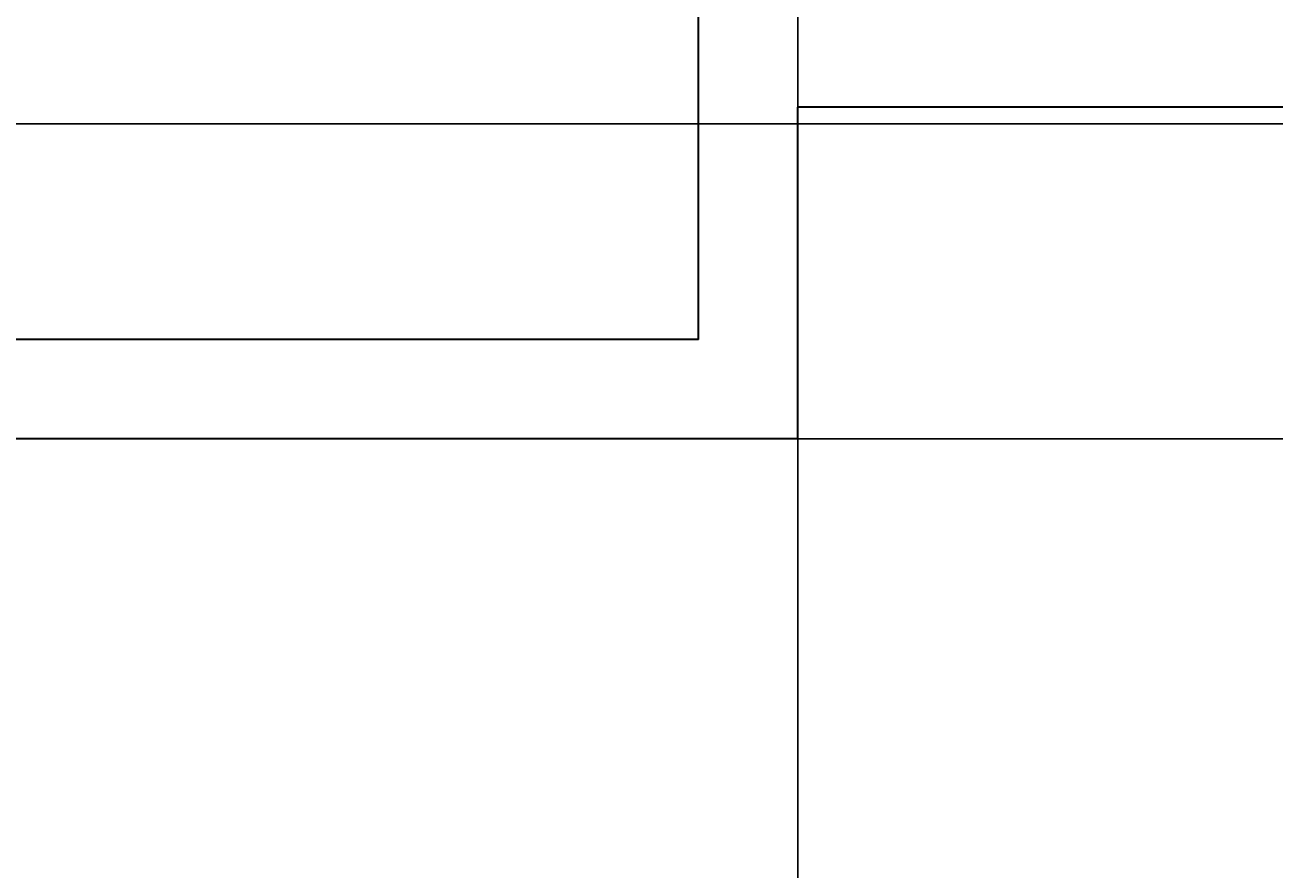
# Model space of a CAD drawing. Units: feet. Extents: x 105 to 1094, y -88 to 588.
# Tile 15 of 59: x 248 to 323, y 250 to 301. Entities that reach past the tile are written whole.
import ezdxf

# ---------------------------------------------------------------- set-up
doc = ezdxf.new("R2010")
doc.units = ezdxf.units.FT
doc.header["$MEASUREMENT"] = 0
doc.layers.add('A-ANNO-DIMS', color=2, linetype='Continuous', lineweight=18)
doc.layers.add('A-WALL', color=7, linetype='Continuous', lineweight=35)
doc.styles.get("Standard").update_dxf_attribs({"font": 'arial.ttf'})
doc.dimstyles.get("Standard").update_dxf_attribs({"dimtxt": 0.18, "dimasz": 0.18, "dimexe": 0.18, "dimexo": 0.0625, "dimgap": 0.09, "dimtad": 0, "dimtih": 1, "dimtoh": 1, "dimdec": 4, "dimzin": 0, "dimdsep": 46, "dimtxsty": 'Standard', "dimcen": 0.09, "dimadec": 0, "dimazin": 0, "dimtfac": 1, "dimtdec": 4, "dimtofl": 0, "dimtmove": 0, "dimatfit": 3, "dimfxl": 1, "dimtolj": 1, "dimtzin": 0, "dimarcsym": 0})

# ---------------------------------------------------------------- blocks, each defined once
blk = doc.blocks.new('*D20')
at = {"layer": 'A-ANNO-DIMS', "color": 0, "lineweight": -2, "transparency": 16777216}
for p, q in [((150.688, 276.019), (150.688, -88.149)), ((1048.688, 276.019), (1048.688, -88.149)), ((150.868, -87.969), (599.399, -87.969)), ((1048.508, -87.969), (599.977, -87.969))]:
    blk.add_line(p, q, dxfattribs=at)
at = {"layer": 'A-ANNO-DIMS', "color": 0, "transparency": 16777216}
for points in [[(150.868, -87.939), (150.868, -87.999), (150.688, -87.969)], [(1048.508, -87.939), (1048.508, -87.999), (1048.688, -87.969)]]:
    blk.add_solid(points, dxfattribs=at)
at = {"layer": 'Defpoints', "color": 0, "transparency": 16777216}
for p in [(150.688, 276.081), (1048.688, 276.081), (1048.688, -87.969)]:
    blk.add_point(p, dxfattribs=at)
at = {"layer": 'A-ANNO-DIMS', "color": 0, "transparency": 16777216, "insert": (599.688, -87.969), "char_height": 0.18, "attachment_point": 5}
blk.add_mtext('\\A1;898', dxfattribs=at)
blk = doc.blocks.new('*D21')
at = {"layer": 'A-ANNO-DIMS', "color": 0, "lineweight": -2, "transparency": 16777216}
for p, q in [((849.626, 543.081), (105.458, 543.081)), ((105.638, 542.901), (105.638, 250.263)), ((105.638, -42.739), (105.638, 249.899)), ((849.626, -42.919), (105.458, -42.919))]:
    blk.add_line(p, q, dxfattribs=at)
at = {"layer": 'A-ANNO-DIMS', "color": 0, "transparency": 16777216}
for points in [[(105.608, 542.901), (105.668, 542.901), (105.638, 543.081)], [(105.608, -42.739), (105.668, -42.739), (105.638, -42.919)]]:
    blk.add_solid(points, dxfattribs=at)
at = {"layer": 'Defpoints', "color": 0, "transparency": 16777216}
for p in [(105.638, 543.081), (849.688, 543.081), (849.688, -42.919)]:
    blk.add_point(p, dxfattribs=at)
at = {"layer": 'A-ANNO-DIMS', "color": 0, "transparency": 16777216, "insert": (105.638, 250.081), "char_height": 0.18, "attachment_point": 5}
blk.add_mtext('\\A1;586', dxfattribs=at)
blk = doc.blocks.new('*D33')
at = {"layer": 'A-ANNO-DIMS', "color": 0, "lineweight": -2, "transparency": 16777216}
for p, q in [((646.626, 395.081), (105.458, 395.081)), ((105.638, 394.901), (105.638, 345.263)), ((105.638, 295.261), (105.638, 344.899)), ((646.626, 295.081), (105.458, 295.081))]:
    blk.add_line(p, q, dxfattribs=at)
at = {"layer": 'A-ANNO-DIMS', "color": 0, "transparency": 16777216}
for points in [[(105.608, 394.901), (105.668, 394.901), (105.638, 395.081)], [(105.608, 295.261), (105.668, 295.261), (105.638, 295.081)]]:
    blk.add_solid(points, dxfattribs=at)
at = {"layer": 'Defpoints', "color": 0, "transparency": 16777216}
for p in [(646.688, 395.081), (105.638, 295.081), (646.688, 295.081)]:
    blk.add_point(p, dxfattribs=at)
at = {"layer": 'A-ANNO-DIMS', "color": 0, "transparency": 16777216, "insert": (105.638, 345.081), "char_height": 0.18, "attachment_point": 5}
blk.add_mtext('\\A1;100', dxfattribs=at)
blk = doc.blocks.new('*D38')
at = {"layer": 'A-ANNO-DIMS', "color": 0, "lineweight": -2, "transparency": 16777216}
for p, q in [((150.688, 224.144), (150.688, 588.311)), ((294.688, 224.144), (294.688, 588.311)), ((150.868, 588.131), (222.408, 588.131)), ((294.508, 588.131), (222.968, 588.131))]:
    blk.add_line(p, q, dxfattribs=at)
at = {"layer": 'A-ANNO-DIMS', "color": 0, "transparency": 16777216}
for points in [[(150.868, 588.161), (150.868, 588.101), (150.688, 588.131)], [(294.508, 588.161), (294.508, 588.101), (294.688, 588.131)]]:
    blk.add_solid(points, dxfattribs=at)
at = {"layer": 'Defpoints', "color": 0, "transparency": 16777216}
for p in [(294.688, 588.131), (150.688, 224.081), (294.688, 224.081)]:
    blk.add_point(p, dxfattribs=at)
at = {"layer": 'A-ANNO-DIMS', "color": 0, "transparency": 16777216, "insert": (222.688, 588.131), "char_height": 0.18, "attachment_point": 5}
blk.add_mtext('\\A1;144', dxfattribs=at)
blk = doc.blocks.new('*D39')
at = {"layer": 'A-ANNO-DIMS', "color": 0, "lineweight": -2, "transparency": 16777216}
for p, q in [((294.688, 204.144), (294.688, 588.311)), ((370.688, 204.144), (370.688, 588.311)), ((294.868, 588.131), (332.47, 588.131)), ((370.508, 588.131), (332.906, 588.131))]:
    blk.add_line(p, q, dxfattribs=at)
at = {"layer": 'A-ANNO-DIMS', "color": 0, "transparency": 16777216}
for points in [[(294.868, 588.161), (294.868, 588.101), (294.688, 588.131)], [(370.508, 588.161), (370.508, 588.101), (370.688, 588.131)]]:
    blk.add_solid(points, dxfattribs=at)
at = {"layer": 'Defpoints', "color": 0, "transparency": 16777216}
for p in [(370.688, 588.131), (294.688, 204.081), (370.688, 204.081)]:
    blk.add_point(p, dxfattribs=at)
at = {"layer": 'A-ANNO-DIMS', "color": 0, "transparency": 16777216, "insert": (332.688, 588.131), "char_height": 0.18, "attachment_point": 5}
blk.add_mtext('\\A1;76', dxfattribs=at)
blk = doc.blocks.new('*D54')
at = {"layer": 'A-ANNO-DIMS', "color": 0, "lineweight": -2, "transparency": 16777216}
for p, q in [((294.751, 296.081), (1093.918, 296.081)), ((1093.738, 295.901), (1093.738, 286.263)), ((1093.738, 276.261), (1093.738, 285.899)), ((294.751, 276.081), (1093.918, 276.081))]:
    blk.add_line(p, q, dxfattribs=at)
at = {"layer": 'A-ANNO-DIMS', "color": 0, "transparency": 16777216}
for points in [[(1093.708, 295.901), (1093.768, 295.901), (1093.738, 296.081)], [(1093.708, 276.261), (1093.768, 276.261), (1093.738, 276.081)]]:
    blk.add_solid(points, dxfattribs=at)
at = {"layer": 'Defpoints', "color": 0, "transparency": 16777216}
for p in [(294.688, 296.081), (1093.738, 296.081), (294.688, 276.081)]:
    blk.add_point(p, dxfattribs=at)
at = {"layer": 'A-ANNO-DIMS', "color": 0, "transparency": 16777216, "insert": (1093.738, 286.081), "char_height": 0.18, "attachment_point": 5}
blk.add_mtext('\\A1;20', dxfattribs=at)

msp = doc.modelspace()

# ---------------------------------------------------------------- linework, layer by layer
at = {"layer": 'A-WALL'}
for p, q in [((288.6883, 282.0812), (288.6883, 320.0812)), ((370.6883, 296.0812), (294.6883, 296.0812)), ((294.6883, 276.0812), (294.6883, 296.0812)), ((288.6883, 282.0812), (156.6883, 282.0812)), ((294.6883, 276.0812), (150.6883, 276.0812))]:
    msp.add_line(p, q, dxfattribs=at)

# ---------------------------------------------------------------- dimensions: what is measured, and where the dimension line sits
at = {"layer": 'A-ANNO-DIMS'}
for base, p1, p2, picture, middle in [((294.6883, 588.1312), (150.6883, 224.0812), (294.6883, 224.0812), '*D38', (222.6883, 588.1312)), ((370.6883, 588.1312), (294.6883, 204.0812), (370.6883, 204.0812), '*D39', (332.6883, 588.1312)), ((1048.6883, -87.9688), (150.6883, 276.0812), (1048.6883, 276.0812), '*D20', (599.6883, -87.9688))]:
    dim = msp.add_linear_dim(base=base, p1=p1, p2=p2, dimstyle='Standard', override={"dimdec": 0, "dimlfac": 1, "dimrnd": 0, "dimzin": 0, "dimdsep": 46, "dimlunit": 2}, dxfattribs=at)
    dim.commit()
    dim.dimension.update_dxf_attribs({"geometry": picture, "text_midpoint": middle})
for base, p1, p2, picture, middle in [((105.6383, 543.0812), (849.6883, -42.9188), (849.6883, 543.0812), '*D21', (105.6383, 250.0812)), ((105.6383, 295.0812), (646.6883, 395.0812), (646.6883, 295.0812), '*D33', (105.6383, 345.0812)), ((1093.7383, 296.0812), (294.6883, 276.0812), (294.6883, 296.0812), '*D54', (1093.7383, 286.0812))]:
    dim = msp.add_linear_dim(base=base, p1=p1, p2=p2, angle=90, dimstyle='Standard', override={"dimdec": 0, "dimlfac": 1, "dimrnd": 0, "dimzin": 0, "dimdsep": 46, "dimlunit": 2}, dxfattribs=at)
    dim.commit()
    dim.dimension.update_dxf_attribs({"geometry": picture, "text_midpoint": middle})

doc.saveas('drawing.dxf')
